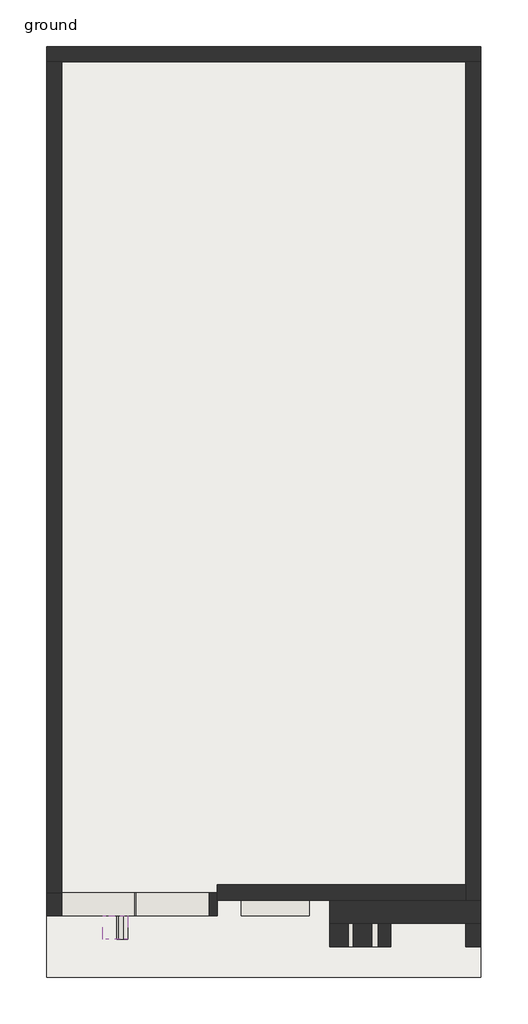
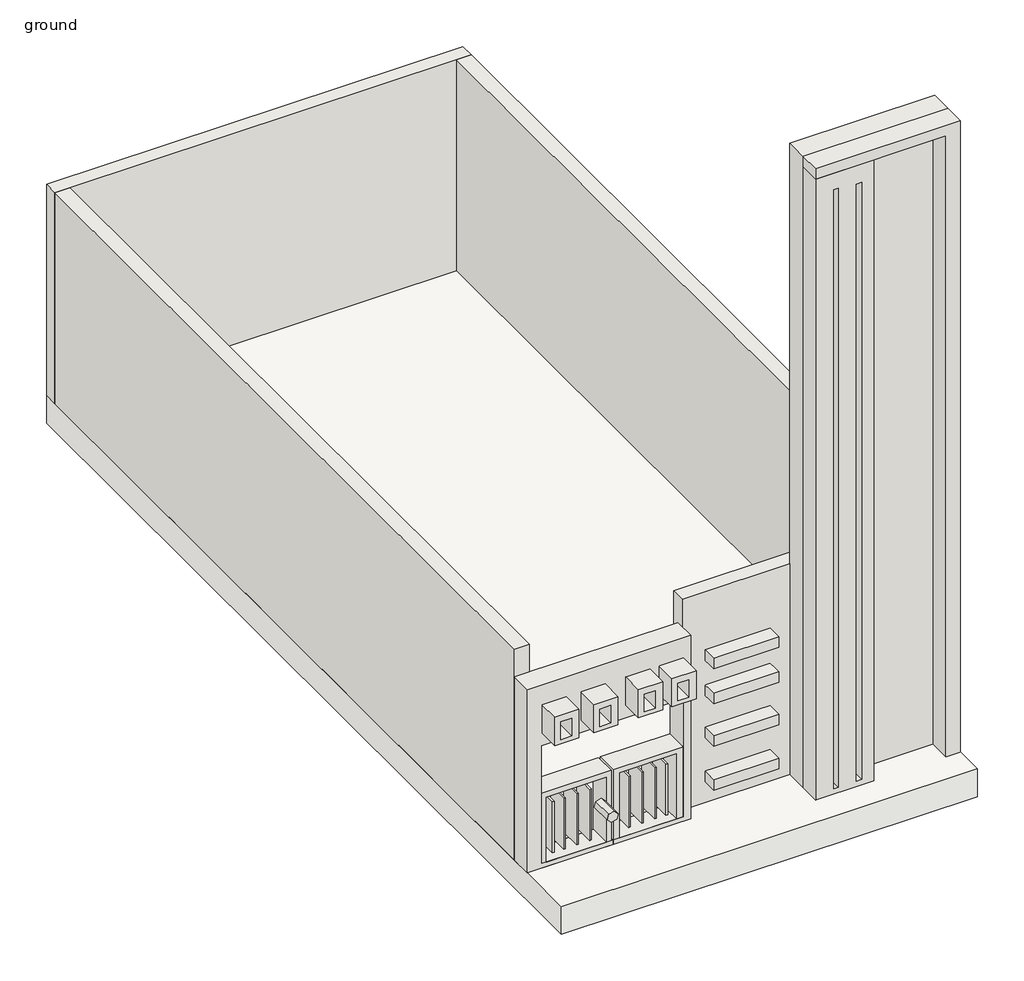
# One storey, incomplete: 12 walls, 1 slab.
"""IFC4 building model written with IfcOpenShell, lengths in millimetres."""

from ifc_helpers import new_model, si_unit, frame, origin, origin_with_axes, place, context, project, spatial, polyline, outline, extrude, faceted_brep, transform, mapped, element, save
from components import walls_1_walls_1_5577fd9e, walls_10_walls_10_47add98f, walls_11_walls_11_7ea3dec3, walls_2_walls_2_973aa2a3, walls_3_walls_3_54e0ac51, walls_4_walls_4_61d7950c, walls_5_walls_5_ae1c99f5, walls_6_walls_6_a828669c

model = new_model("IFC4")

# Units and contexts
model_context = context("Model", 3, world=origin())
ifc_project = project(units=[si_unit("LENGTHUNIT", "METRE", prefix="MILLI")], contexts=[model_context])

# Site, building, storey
site = spatial("IfcSite", under=ifc_project)
building = spatial("IfcBuilding", under=site)
storey = spatial("IfcBuildingStorey", under=building, Name="ground", Elevation=0.0)

# Slab
placement = place(None, origin())
element("IfcSlab", 1, ObjectType="Generic Floor - 400mm", at=placement, inside=storey, context=model_context, shape_type="SweptSolid", body=[
    extrude(outline(polyline([(-4193.9407032, 15033.7956099), (-4193.9407032, 2849.7255409), (-9880.3407032, 2849.7255409), (-9880.3407032, 15033.7956099), (-4193.9407032, 15033.7956099)])), frame((0.0, 0.0, -400.0), z_axis=(0.0, 0.0, 1.0), x_axis=(1.0, 0.0, 0.0)), (0.0, 0.0, 1.0), 400.0),
])

# Walls
element("IfcWall", 2, ObjectType="Generic - 9\"", at=placement, inside=storey, context=model_context, shape_type="Brep", body=[
    faceted_brep([(-9880.3407032, 14833.7956099, 0.0), (-9680.3407032, 14833.7956099, 0.0), (-4393.9407032, 14833.7956099, 0.0), (-4193.9407032, 14833.7956099, 0.0), (-4193.9407032, 14833.7956099, 3048.0), (-4393.9407032, 14833.7956099, 3048.0), (-9680.3407032, 14833.7956099, 3048.0), (-9880.3407032, 14833.7956099, 3048.0), (-9880.3407032, 15033.7956099, 0.0), (-9880.3407032, 15033.7956099, 3048.0), (-4193.9407032, 15033.7956099, 3048.0), (-4193.9407032, 15033.7956099, 0.0)], [[[0, 1, 2, 3, 4, 5, 6, 7]], [[8, 9, 10, 11]], [[3, 2, 1, 0, 8, 11]], [[7, 6, 5, 4, 10, 9]], [[4, 3, 11, 10]], [[0, 7, 9, 8]]]),
])
element("IfcWall", 3, ObjectType="Generic - 9\"", at=placement, inside=storey, context=model_context, shape_type="Brep", body=[
    faceted_brep([(-4393.9407032, 14833.7956099, 0.0), (-4393.9407032, 4060.9956099, 0.0), (-4393.9407032, 3860.9956099, 0.0), (-4393.9407032, 3860.9956099, 3048.0), (-4393.9407032, 4060.9956099, 3048.0), (-4393.9407032, 14833.7956099, 3048.0), (-4193.9407032, 14833.7956099, 0.0), (-4193.9407032, 14833.7956099, 3048.0), (-4193.9407032, 3860.9956099, 3048.0), (-4193.9407032, 3860.9956099, 0.0)], [[[0, 1, 2, 3, 4, 5]], [[6, 7, 8, 9]], [[2, 1, 0, 6, 9]], [[5, 4, 3, 8, 7]], [[0, 5, 7, 6]], [[3, 2, 9, 8]]]),
])
element("IfcWall", 4, ObjectType="Generic - 9\"", at=placement, inside=storey, context=model_context, shape_type="SweptSolid", body=[
    extrude(outline(polyline([(-7646.7407032, 4060.9956099), (-4393.9407032, 4060.9956099), (-4393.9407032, 3860.9956099), (-7646.7407032, 3860.9956099), (-7646.7407032, 4060.9956099)])), origin_with_axes(), (0.0, 0.0, 1.0), 3048.0),
])
element("IfcWall", 5, ObjectType="Generic - 9\"", at=placement, inside=storey, context=model_context, shape_type="SweptSolid", body=[
    extrude(outline(polyline([(-9680.3407032, 14833.7956099), (-9680.3407032, 3960.9956099), (-9880.3407032, 3960.9956099), (-9880.3407032, 14833.7956099), (-9680.3407032, 14833.7956099)])), origin_with_axes(), (0.0, 0.0, 1.0), 3048.0),
])
walls_1_walls_1_shape = walls_1_walls_1_5577fd9e(model_context)
element("IfcWall", 6, ObjectType="Walls 1 : Walls 1", at=placement, inside=storey, context=model_context, shape_type="MappedRepresentation", body=[
    mapped(walls_1_walls_1_shape, transform((0.0, 0.0, 0.0), x_axis=(1.0, 0.0, 0.0), y_axis=(0.0, 1.0, 0.0), z_axis=(0.0, 0.0, 1.0))),
])
walls_10_walls_10_shape = walls_10_walls_10_47add98f(model_context)
element("IfcWall", 7, ObjectType="Walls 10 : Walls 10", at=placement, inside=storey, context=model_context, shape_type="MappedRepresentation", body=[
    mapped(walls_10_walls_10_shape, transform((0.0, 0.0, 0.0), x_axis=(1.0, 0.0, 0.0), y_axis=(0.0, 1.0, 0.0), z_axis=(0.0, 0.0, 1.0))),
])
walls_11_walls_11_shape = walls_11_walls_11_7ea3dec3(model_context)
element("IfcWall", 8, ObjectType="Walls 11 : Walls 11", at=placement, inside=storey, context=model_context, shape_type="MappedRepresentation", body=[
    mapped(walls_11_walls_11_shape, transform((0.0, 0.0, 0.0), x_axis=(1.0, 0.0, 0.0), y_axis=(0.0, 1.0, 0.0), z_axis=(0.0, 0.0, 1.0))),
])
walls_2_walls_2_shape = walls_2_walls_2_973aa2a3(model_context)
element("IfcWall", 9, ObjectType="Walls 2 : Walls 2", at=placement, inside=storey, context=model_context, shape_type="MappedRepresentation", body=[
    mapped(walls_2_walls_2_shape, transform((0.0, 0.0, 0.0), x_axis=(1.0, 0.0, 0.0), y_axis=(0.0, 1.0, 0.0), z_axis=(0.0, 0.0, 1.0))),
])
walls_3_walls_3_shape = walls_3_walls_3_54e0ac51(model_context)
element("IfcWall", 10, ObjectType="Walls 3 : Walls 3", at=placement, inside=storey, context=model_context, shape_type="MappedRepresentation", body=[
    mapped(walls_3_walls_3_shape, transform((0.0, 0.0, 0.0), x_axis=(1.0, 0.0, 0.0), y_axis=(0.0, 1.0, 0.0), z_axis=(0.0, 0.0, 1.0))),
])
walls_4_walls_4_shape = walls_4_walls_4_61d7950c(model_context)
element("IfcWall", 11, ObjectType="Walls 4 : Walls 4", at=placement, inside=storey, context=model_context, shape_type="MappedRepresentation", body=[
    mapped(walls_4_walls_4_shape, transform((0.0, 0.0, 0.0), x_axis=(1.0, 0.0, 0.0), y_axis=(0.0, 1.0, 0.0), z_axis=(0.0, 0.0, 1.0))),
])
walls_5_walls_5_shape = walls_5_walls_5_ae1c99f5(model_context)
element("IfcWall", 12, ObjectType="Walls 5 : Walls 5", at=placement, inside=storey, context=model_context, shape_type="MappedRepresentation", body=[
    mapped(walls_5_walls_5_shape, transform((0.0, 0.0, 0.0), x_axis=(1.0, 0.0, 0.0), y_axis=(0.0, 1.0, 0.0), z_axis=(0.0, 0.0, 1.0))),
])
walls_6_walls_6_shape = walls_6_walls_6_a828669c(model_context)
element("IfcWall", 13, ObjectType="Walls 6 : Walls 6", at=placement, inside=storey, context=model_context, shape_type="MappedRepresentation", body=[
    mapped(walls_6_walls_6_shape, transform((0.0, 0.0, 0.0), x_axis=(1.0, 0.0, 0.0), y_axis=(0.0, 1.0, 0.0), z_axis=(0.0, 0.0, 1.0))),
])

save(model, "model.ifc")

# Revit data of these elements
# Type "Generic Floor - 400mm"
#   Function = 0
#   Layers, outside or top first: 400 mm no material (function 1)
# Type "Generic - 9\""
#   Layers, outside or top first: 200 mm no material (function 1)
# Element 1 (IfcSlab, "Generic Floor - 400mm")
#   Height Offset From Level = 0 mm
#   Phase Created = New Construction
#   Materials on its faces: "Default Roof"
# Elements 2, 3, 4, 5 (IfcWall, "Generic - 9\"")
#   Top Offset = 0 mm
#   Base Offset = 0 mm
#   Unconnected Height = 3048 mm
#   wall height = 3048 mm
#   Phase Created = New Construction
#   Base Constraint = ground
#   Materials on its faces: "Default Wall"
# Element 6 (IfcWall, "Walls 1 : Walls 1")
#   Phase Created = New Construction
#   Materials on its faces: "Default Wall"
# Element 7 (IfcWall, "Walls 10 : Walls 10")
#   Phase Created = New Construction
#   Materials on its faces: "Default Wall"
# Element 8 (IfcWall, "Walls 11 : Walls 11")
#   Phase Created = New Construction
#   Materials on its faces: "Default Wall"
# Element 9 (IfcWall, "Walls 2 : Walls 2")
#   Phase Created = New Construction
#   Materials on its faces: "Default Wall"
# Element 10 (IfcWall, "Walls 3 : Walls 3")
#   Phase Created = New Construction
#   Materials on its faces: "Default Wall"
# Element 11 (IfcWall, "Walls 4 : Walls 4")
#   Phase Created = New Construction
#   Materials on its faces: "Default Wall"
# Element 12 (IfcWall, "Walls 5 : Walls 5")
#   Phase Created = New Construction
#   Materials on its faces: "Default Wall"
# Element 13 (IfcWall, "Walls 6 : Walls 6")
#   Phase Created = New Construction
#   Materials on its faces: "Default Wall"
# Materials
#   "Default Roof": colour RGB 80 80 80, transparency 0
#   "Default Wall": colour RGB 80 80 80, transparency 0
